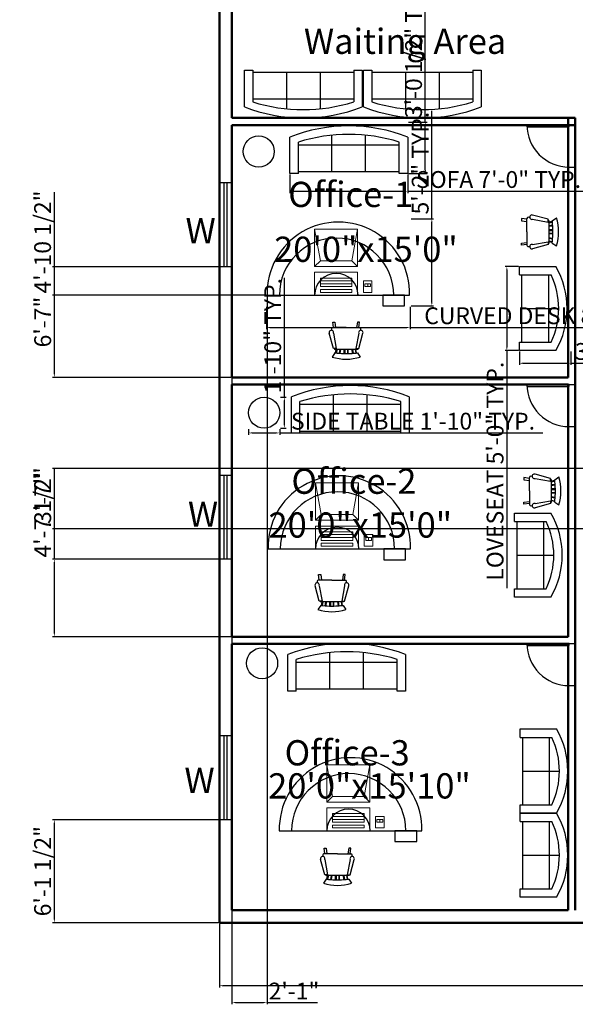
# Model space of a CAD drawing. Units: inches. Extents: x 1953 to 3378, y 1378 to 2530.
# Tile 1 of 5: x 1953 to 2350, y 1388 to 2090. Entities that reach past the tile are written whole.
import ezdxf

# ---------------------------------------------------------------- set-up
doc = ezdxf.new("R2010")
doc.units = ezdxf.units.IN
for name, color, linetype, lineweight in [('A-ANNO-DIMS', 2, 'Continuous', 18), ('A-ANNO-TEXT', 7, 'Continuous', 18), ('A-AREA-IDEN', 4, 'Continuous', 18), ('A-DOOR', 4, 'Continuous', 25), ('A-EQPM', 50, 'Continuous', 18), ('A-FURN', 50, 'Continuous', 25), ('wall', 7, 'Continuous', 50), ('windows', 180, 'Continuous', 25)]:
    doc.layers.add(name, color=color, linetype=linetype, lineweight=lineweight)
doc.styles.get("Standard").update_dxf_attribs({"font": 'arial.ttf'})
doc.dimstyles.new('ISO-25', dxfattribs={"dimtxt": 12, "dimasz": 2.5, "dimexe": 1.25, "dimexo": 0.625, "dimtad": 1, "dimdec": 1, "dimlunit": 4, "dimtxsty": 'Standard', "dimcen": 2.5, "dimadec": 0, "dimazin": 0, "dimtfac": 1, "dimtdec": 1, "dimtmove": 0, "dimatfit": 3, "dimfxl": 1, "dimarcsym": 0})

# ---------------------------------------------------------------- blocks, each defined once
blk = doc.blocks.new('*U10')
for p, q in [((0, 0), (0, 6)), ((40, 0), (40, 6))]:
    blk.add_line(p, q)
blk.add_lwpolyline([(0, 0), (0, -40), (1.75, -40), (1.75, 0)], close=True)
blk.add_arc((0, 0), 40, 270, 0)
blk = doc.blocks.new('*U9')
for p, q in [((0, 0), (0, 6)), ((40, 0), (40, 6))]:
    blk.add_line(p, q)
blk.add_lwpolyline([(0, 0), (0, -40), (1.75, -40), (1.75, 0)], close=True)
blk.add_arc((0, 0), 40, 270, 0)
blk = doc.blocks.new('*U8')
for p, q in [((0, 0), (0, 6)), ((40, 0), (40, 6))]:
    blk.add_line(p, q)
blk.add_lwpolyline([(0, 0), (0, -40), (1.75, -40), (1.75, 0)], close=True)
blk.add_arc((0, 0), 40, 270, 360)
blk = doc.blocks.new('Sofa - Roundback 7 ft.')
for p, q in [((-12.00002, -32.4421), (-12.00003, -6.5971)), ((11.99997, -32.4421), (11.99998, -6.5971)), ((-36.000027, -34), (-36.000027, -11.4696)), ((-35.999844, -13.3819), (35.9998, -13.3819)), ((35.99998, -34), (35.99998, -11.4696)), ((-36.000027, -32.4421), (35.99998, -32.4421))]:
    blk.add_line(p, q)
for points in [[(-36.000027, -34), (-42.000027, -34), (-42.000027, -8)], [(41.99998, -8), (41.99998, -34), (35.99998, -34)]]:
    blk.add_lwpolyline(points)
for centre, radius, start, end in [((0, -114.25), 114.25, 68.43141, 111.5686), ((-0.00001, -127.1968), 121.1968, 72.72033, 107.2797)]:
    blk.add_arc(centre, radius, start, end)
blk = doc.blocks.new('Computer Terminal')
for p, q in [((-10, 11.5), (5, 11.5)), ((-8, 0.5), (-10, 11.5)), ((-10, -1.5), (-10, 11.5)), ((5, 11.5), (3, 0.5)), ((5, 11.5), (5, -1.5)), ((-10, -1.5), (-8, 0.5)), ((3, 0.5), (-8, 0.5)), ((3, 0.5), (5, -1.5)), ((5, -1.5), (-10, -1.5)), ((-10, -11.5), (-10, -3.5)), ((-10, -3.5), (5, -3.5)), ((-8, -5.5), (-8, -8.5)), ((3, -5.5), (-8, -5.5)), ((3, -6.5), (-8, -6.5)), ((3, -8.5), (3, -5.5)), ((5, -3.5), (5, -11.5)), ((10, -6.5), (7, -6.5)), ((7, -6.5), (7, -10.5)), ((10, -10.5), (10, -6.5)), ((-8, -7.5), (3, -7.5)), ((-8, -8.5), (3, -8.5)), ((-8, -9.5), (-8, -10.5)), ((3, -9.5), (-8, -9.5)), ((3, -10.5), (3, -9.5)), ((9.5, -7.5), (7.5, -7.5)), ((7.5, -7.5), (7.5, -8.5)), ((7.5, -8.5), (9.5, -8.5)), ((8.5, -7.5), (8.5, -8.5)), ((9.5, -8.5), (9.5, -7.5)), ((5, -11.5), (-10, -11.5)), ((-8, -10.5), (3, -10.5)), ((7, -10.5), (10, -10.5))]:
    blk.add_line(p, q)
blk = doc.blocks.new('Chair - Rocking')
for p, q in [((-8, -4.5), (-10, -1.5)), ((-8.23428, -6.99939), (-8.3093, -7.47958)), ((-8.23041, -7), (8.23915, -7)), ((-7.5, -4.5), (-7, -7)), ((-6.5, -7), (-7.02225, -4.43)), ((-4.5, -7), (-4.96674, -4.19951)), ((-4, -7), (-4.40532, -4.16272)), ((-1.5, -4.05012), (-1.5, -7)), ((-1, -7), (-1, -4.05012)), ((1, -7), (1, -4.04655)), ((1.5, -4.05012), (1.5, -7)), ((4, -7), (4.40187, -4.18694)), ((4.5, -7), (4.96761, -4.19437)), ((6.5, -7), (7, -4.4057)), ((7.5, -4.5), (7, -7)), ((8, -4.5), (10, -1.5)), ((8.31071, -7.48854), (8.23449, -7.00073)), ((-9, -7.5), (-12, -18.49999)), ((-7, -7.5), (-9, -7.5)), ((-9, -18.49999), (-7, -7.5)), ((7, -7.5), (9, -7.5)), ((9, -18.49999), (7, -7.5)), ((9, -7.5), (12, -18.49999)), ((-10.36644, -20.64523), (-10.5, -21.49999)), ((10.5, -21.49999), (10.3575, -20.58798)), ((-9, -22.49999), (-9.5, -26.49999)), ((0, -22.49999), (-9.5, -22.49999)), ((-9.5, -26.49999), (-8, -26.49999)), ((-8, -26.49999), (-7.5, -22.49999)), ((0, -22.49999), (9.5, -22.49999)), ((8, -26.49999), (7.5, -22.49999)), ((9.5, -26.49999), (8, -26.49999)), ((9, -22.49999), (9.5, -26.49999))]:
    blk.add_line(p, q)
for centre, radius, start, end in [((0, -34.08333), 34.08333, 72.93847, 107.0615), ((0, -68.25004), 64.25, 93.92211, 97.15267), ((0, -68.25004), 64.25, 82.84733, 93.92211), ((-10.5, -18.99999), 1.58114, 161.5651, 18.43495), ((10.5, -18.99999), 1.58114, 161.5651, 18.43495), ((-9.5, -21.49999), 1, 180, 270), ((9.5, -21.49999), 1, 270, 0)]:
    blk.add_arc(centre, radius, start, end)
blk = doc.blocks.new('Sofa - Roundback Loveseat 5 ft.')
for p, q in [((0, -32.44198), (0, -5.99998)), ((-24, -33.99998), (-24, -11.46958)), ((-23.9998, -13.38178), (23.99986, -13.38178)), ((24.00004, -33.99998), (24.00004, -11.46958)), ((-24, -32.44198), (24.00004, -32.44198))]:
    blk.add_line(p, q)
for points in [[(-24, -33.99998), (-30, -33.99998), (-30, -7.99998)], [(30.00004, -7.99998), (30.00004, -33.99998), (24.00004, -33.99998)]]:
    blk.add_lwpolyline(points)
for centre, radius, start, end in [((0, -60.24998), 60.24998, 60.13715, 119.8628), ((0, -61.38438), 55.38444, 64.32083, 115.6792)]:
    blk.add_arc(centre, radius, start, end)
blk = doc.blocks.new('*D28')
at = {"layer": 'A-ANNO-DIMS', "color": 0, "lineweight": -2, "transparency": 16777216}
for p, q in [((2095.75, 1445.39), (2095.75, 1399.8)), ((2695.75, 1445.39), (2695.75, 1399.8)), ((2693.25, 1401.05), (2098.25, 1401.05))]:
    blk.add_line(p, q, dxfattribs=at)
at = {"layer": 'A-ANNO-DIMS', "color": 0, "transparency": 16777216}
for points in [[(2098.25, 1401.47), (2098.25, 1400.63), (2095.75, 1401.05)], [(2693.25, 1401.47), (2693.25, 1400.63), (2695.75, 1401.05)]]:
    blk.add_solid(points, dxfattribs=at)
at = {"layer": 'Defpoints', "color": 0, "transparency": 16777216}
for p in [(2095.75, 1446.01), (2695.75, 1446.01), (2095.75, 1401.05)]:
    blk.add_point(p, dxfattribs=at)
at = {"layer": 'A-ANNO-DIMS', "color": 0, "transparency": 16777216, "insert": (2395.75, 1407.8), "char_height": 12, "attachment_point": 5}
blk.add_mtext("50'", dxfattribs=at)
blk = doc.blocks.new('WINDOW-60IN')
for p, q in [((0, 5.5), (60, 5.5)), ((0, 5.5), (60, 5.5)), ((0, 3.5), (60, 3.5))]:
    blk.add_line(p, q)
blk.add_lwpolyline([(0, 9), (60, 9), (60, 0), (0, 0)], close=True)
blk = doc.blocks.new('DESK-SEMICIRCULAR')
blk.add_line((0.02, 7.63), (101.66, 7.63))
blk.add_lwpolyline([(82.57, 7.63), (82.57, 0), (98.08, 0), (98.08, 7.63)], close=True)
for centre, radius, start, end in [((50.84, 8.97), 50.84, 358.48644, 181.51356), ((49.55, 7.63), 40.78, 0, 180), ((49.41, 7.63), 15.51, 0, 180)]:
    blk.add_arc(centre, radius, start, end)
blk = doc.blocks.new('SIDE-TABLE-ROUND')
blk.add_circle((11.1, 11.1), 11.1)
blk = doc.blocks.new('*D40')
at = {"layer": 'A-ANNO-DIMS', "color": 0, "lineweight": -2, "transparency": 16777216}
for p, q in [((2309.27, 1914.09), (2299.64, 1914.09)), ((2300.89, 1911.59), (2300.89, 1856.59)), ((2309.27, 1854.09), (2299.64, 1854.09)), ((2300.89, 1854.09), (2300.89, 1684.55))]:
    blk.add_line(p, q, dxfattribs=at)
at = {"layer": 'A-ANNO-DIMS', "color": 0, "transparency": 16777216}
for points in [[(2300.47, 1911.59), (2301.31, 1911.59), (2300.89, 1914.09)], [(2300.47, 1856.59), (2301.31, 1856.59), (2300.89, 1854.09)]]:
    blk.add_solid(points, dxfattribs=at)
at = {"layer": 'Defpoints', "color": 0, "transparency": 16777216}
for p in [(2309.89, 1914.09), (2300.89, 1854.09), (2309.89, 1854.09)]:
    blk.add_point(p, dxfattribs=at)
at = {"layer": 'A-ANNO-DIMS', "color": 0, "transparency": 16777216, "insert": (2294.06, 1768.07), "char_height": 12, "attachment_point": 5, "rotation": 90}
blk.add_mtext('LOVESEAT 5\'-0" TYP.', dxfattribs=at)
blk = doc.blocks.new('*D41')
at = {"layer": 'A-ANNO-DIMS', "color": 0, "lineweight": -2, "transparency": 16777216}
for p, q in [((2309.89, 1853.46), (2309.89, 1843.84)), ((2346.56, 1853.46), (2346.56, 1843.84)), ((2312.39, 1845.09), (2344.06, 1845.09)), ((2346.56, 1845.09), (2451.41, 1845.09))]:
    blk.add_line(p, q, dxfattribs=at)
at = {"layer": 'A-ANNO-DIMS', "color": 0, "transparency": 16777216}
for points in [[(2312.39, 1845.5), (2312.39, 1844.67), (2309.89, 1845.09)], [(2344.06, 1845.5), (2344.06, 1844.67), (2346.56, 1845.09)]]:
    blk.add_solid(points, dxfattribs=at)
at = {"layer": 'Defpoints', "color": 0, "transparency": 16777216}
for p in [(2309.89, 1854.09), (2346.56, 1854.09), (2346.56, 1845.09)]:
    blk.add_point(p, dxfattribs=at)
at = {"layer": 'A-ANNO-DIMS', "color": 0, "transparency": 16777216, "insert": (2400.23, 1851.92), "char_height": 12, "attachment_point": 5}
blk.add_mtext('3\'-0 1/2" TYP.', dxfattribs=at)
blk = doc.blocks.new('*D42')
at = {"layer": 'A-ANNO-DIMS', "color": 0, "lineweight": -2, "transparency": 16777216}
for p, q in [((2146.13, 1979.72), (2146.13, 1966.49)), ((2230.13, 1979.72), (2230.13, 1966.49)), ((2148.63, 1967.74), (2227.63, 1967.74)), ((2230.13, 1967.74), (2357.26, 1967.74))]:
    blk.add_line(p, q, dxfattribs=at)
at = {"layer": 'A-ANNO-DIMS', "color": 0, "transparency": 16777216}
for points in [[(2148.63, 1968.16), (2148.63, 1967.33), (2146.13, 1967.74)], [(2227.63, 1968.16), (2227.63, 1967.33), (2230.13, 1967.74)]]:
    blk.add_solid(points, dxfattribs=at)
at = {"layer": 'Defpoints', "color": 0, "transparency": 16777216}
for p in [(2146.13, 1980.34), (2230.13, 1980.34), (2230.13, 1967.74)]:
    blk.add_point(p, dxfattribs=at)
at = {"layer": 'A-ANNO-DIMS', "color": 0, "transparency": 16777216, "insert": (2294.95, 1974.58), "char_height": 12, "attachment_point": 5}
blk.add_mtext('SOFA 7\'-0" TYP.', dxfattribs=at)
blk = doc.blocks.new('*D43')
at = {"layer": 'A-ANNO-DIMS', "color": 0, "lineweight": -2, "transparency": 16777216}
for p, q in [((2242.73, 2017.01), (2242.73, 2121.86)), ((2230.75, 2017.01), (2243.98, 2017.01)), ((2242.73, 1982.84), (2242.73, 2014.51)), ((2230.75, 1980.34), (2243.98, 1980.34))]:
    blk.add_line(p, q, dxfattribs=at)
at = {"layer": 'A-ANNO-DIMS', "color": 0, "transparency": 16777216}
for points in [[(2242.31, 2014.51), (2243.14, 2014.51), (2242.73, 2017.01)], [(2242.31, 1982.84), (2243.14, 1982.84), (2242.73, 1980.34)]]:
    blk.add_solid(points, dxfattribs=at)
at = {"layer": 'Defpoints', "color": 0, "transparency": 16777216}
for p in [(2230.13, 2017.01), (2242.73, 2017.01), (2230.13, 1980.34)]:
    blk.add_point(p, dxfattribs=at)
at = {"layer": 'A-ANNO-DIMS', "color": 0, "transparency": 16777216, "insert": (2235.89, 2070.69), "char_height": 12, "attachment_point": 5, "rotation": 90}
blk.add_mtext('3\'-0 1/2" TYP.', dxfattribs=at)
blk = doc.blocks.new('*D44')
at = {"layer": 'A-ANNO-DIMS', "color": 0, "lineweight": -2, "transparency": 16777216}
for p, q in [((2129.36, 1885.33), (2129.36, 1869.31)), ((2231.98, 1885.33), (2231.98, 1869.31)), ((2131.86, 1870.56), (2229.48, 1870.56)), ((2231.98, 1870.56), (2462.45, 1870.56))]:
    blk.add_line(p, q, dxfattribs=at)
at = {"layer": 'A-ANNO-DIMS', "color": 0, "transparency": 16777216}
for points in [[(2131.86, 1870.98), (2131.86, 1870.14), (2129.36, 1870.56)], [(2229.48, 1870.98), (2229.48, 1870.14), (2231.98, 1870.56)]]:
    blk.add_solid(points, dxfattribs=at)
at = {"layer": 'Defpoints', "color": 0, "transparency": 16777216}
for p in [(2129.36, 1885.95), (2231.98, 1885.95), (2231.98, 1870.56)]:
    blk.add_point(p, dxfattribs=at)
at = {"layer": 'A-ANNO-DIMS', "color": 0, "transparency": 16777216, "insert": (2348.46, 1877.39), "char_height": 12, "attachment_point": 5}
blk.add_mtext('CURVED DESK 8\'-6 1/2" TYP.', dxfattribs=at)
blk = doc.blocks.new('*D45')
at = {"layer": 'A-ANNO-DIMS', "color": 0, "lineweight": -2, "transparency": 16777216}
for p, q in [((2247.37, 1948.11), (2247.37, 2025.01)), ((2232.6, 1948.11), (2248.62, 1948.11)), ((2247.37, 1888.45), (2247.37, 1945.61)), ((2232.6, 1885.95), (2248.62, 1885.95))]:
    blk.add_line(p, q, dxfattribs=at)
at = {"layer": 'A-ANNO-DIMS', "color": 0, "transparency": 16777216}
for points in [[(2246.96, 1945.61), (2247.79, 1945.61), (2247.37, 1948.11)], [(2246.96, 1888.45), (2247.79, 1888.45), (2247.37, 1885.95)]]:
    blk.add_solid(points, dxfattribs=at)
at = {"layer": 'Defpoints', "color": 0, "transparency": 16777216}
for p in [(2231.98, 1948.11), (2247.37, 1948.11), (2231.98, 1885.95)]:
    blk.add_point(p, dxfattribs=at)
at = {"layer": 'A-ANNO-DIMS', "color": 0, "transparency": 16777216, "insert": (2240.62, 1987.81), "char_height": 12, "attachment_point": 5, "rotation": 90}
blk.add_mtext('5\'-2" TYP.', dxfattribs=at)
blk = doc.blocks.new('*D48')
at = {"layer": 'A-ANNO-DIMS', "color": 0, "lineweight": -2, "transparency": 16777216}
for p, q in [((2116.61, 1798.07), (2116.61, 1794.11)), ((2138.81, 1798.07), (2138.81, 1794.11)), ((2119.11, 1795.36), (2136.31, 1795.36)), ((2138.81, 1795.36), (2326.52, 1795.36))]:
    blk.add_line(p, q, dxfattribs=at)
at = {"layer": 'A-ANNO-DIMS', "color": 0, "transparency": 16777216}
for points in [[(2119.11, 1795.78), (2119.11, 1794.95), (2116.61, 1795.36)], [(2136.31, 1795.78), (2136.31, 1794.95), (2138.81, 1795.36)]]:
    blk.add_solid(points, dxfattribs=at)
at = {"layer": 'Defpoints', "color": 0, "transparency": 16777216}
for p in [(2116.61, 1798.69), (2138.81, 1798.69), (2138.81, 1795.36)]:
    blk.add_point(p, dxfattribs=at)
at = {"layer": 'A-ANNO-DIMS', "color": 0, "transparency": 16777216, "insert": (2233.92, 1802.19), "char_height": 12, "attachment_point": 5}
blk.add_mtext('SIDE TABLE 1\'-10" TYP.', dxfattribs=at)
blk = doc.blocks.new('*D49')
at = {"layer": 'A-ANNO-DIMS', "color": 0, "lineweight": -2, "transparency": 16777216}
for p, q in [((2142.14, 1820.89), (2142.14, 1905.98)), ((2139.44, 1820.89), (2143.39, 1820.89)), ((2142.14, 1801.19), (2142.14, 1818.39)), ((2139.44, 1798.69), (2143.39, 1798.69))]:
    blk.add_line(p, q, dxfattribs=at)
at = {"layer": 'A-ANNO-DIMS', "color": 0, "transparency": 16777216}
for points in [[(2141.72, 1818.39), (2142.56, 1818.39), (2142.14, 1820.89)], [(2141.72, 1801.19), (2142.56, 1801.19), (2142.14, 1798.69)]]:
    blk.add_solid(points, dxfattribs=at)
at = {"layer": 'Defpoints', "color": 0, "transparency": 16777216}
for p in [(2138.81, 1820.89), (2142.14, 1820.89), (2138.81, 1798.69)]:
    blk.add_point(p, dxfattribs=at)
at = {"layer": 'A-ANNO-DIMS', "color": 0, "transparency": 16777216, "insert": (2135.39, 1864.69), "char_height": 12, "attachment_point": 5, "rotation": 90}
blk.add_mtext('1\'-10" TYP.', dxfattribs=at)
blk = doc.blocks.new('*D66')
at = {"layer": 'A-ANNO-DIMS', "color": 0, "lineweight": -2, "transparency": 16777216}
for p, q in [((2095.12, 1519.49), (1976.77, 1519.49)), ((1978.02, 1448.51), (1978.02, 1516.99)), ((2095.12, 1446.01), (1976.77, 1446.01))]:
    blk.add_line(p, q, dxfattribs=at)
at = {"layer": 'A-ANNO-DIMS', "color": 0, "transparency": 16777216}
for points in [[(1977.6, 1516.99), (1978.44, 1516.99), (1978.02, 1519.49)], [(1977.6, 1448.51), (1978.44, 1448.51), (1978.02, 1446.01)]]:
    blk.add_solid(points, dxfattribs=at)
at = {"layer": 'Defpoints', "color": 0, "transparency": 16777216}
for p in [(1978.02, 1519.49), (2095.75, 1519.49), (2095.75, 1446.01)]:
    blk.add_point(p, dxfattribs=at)
at = {"layer": 'A-ANNO-DIMS', "color": 0, "transparency": 16777216, "insert": (1971.19, 1482.75), "char_height": 12, "attachment_point": 5, "rotation": 90}
blk.add_mtext('6\'-1 1/2"', dxfattribs=at)
blk = doc.blocks.new('*D67')
at = {"layer": 'A-ANNO-DIMS', "color": 0, "lineweight": -2, "transparency": 16777216}
for p, q in [((1978.02, 1705.35), (1978.02, 1769.45)), ((2104.12, 1705.35), (1976.77, 1705.35)), ((1978.02, 1652.51), (1978.02, 1702.85)), ((2104.12, 1650.01), (1976.77, 1650.01))]:
    blk.add_line(p, q, dxfattribs=at)
at = {"layer": 'A-ANNO-DIMS', "color": 0, "transparency": 16777216}
for points in [[(1977.6, 1702.85), (1978.44, 1702.85), (1978.02, 1705.35)], [(1977.6, 1652.51), (1978.44, 1652.51), (1978.02, 1650.01)]]:
    blk.add_solid(points, dxfattribs=at)
at = {"layer": 'Defpoints', "color": 0, "transparency": 16777216}
for p in [(1978.02, 1705.35), (2104.75, 1705.35), (2104.75, 1650.01)]:
    blk.add_point(p, dxfattribs=at)
at = {"layer": 'A-ANNO-DIMS', "color": 0, "transparency": 16777216, "insert": (1971.19, 1738.65), "char_height": 12, "attachment_point": 5, "rotation": 90}
blk.add_mtext('4\'-7 1/2"', dxfattribs=at)
blk = doc.blocks.new('*D68')
at = {"layer": 'A-ANNO-DIMS', "color": 0, "lineweight": -2, "transparency": 16777216}
for p, q in [((2104.12, 1913.91), (1976.77, 1913.91)), ((1978.02, 1837.51), (1978.02, 1911.41)), ((2104.12, 1835.01), (1976.77, 1835.01))]:
    blk.add_line(p, q, dxfattribs=at)
at = {"layer": 'A-ANNO-DIMS', "color": 0, "transparency": 16777216}
for points in [[(1977.6, 1911.41), (1978.44, 1911.41), (1978.02, 1913.91)], [(1977.6, 1837.51), (1978.44, 1837.51), (1978.02, 1835.01)]]:
    blk.add_solid(points, dxfattribs=at)
at = {"layer": 'Defpoints', "color": 0, "transparency": 16777216}
for p in [(1978.02, 1913.91), (2104.75, 1913.91), (2104.75, 1835.01)]:
    blk.add_point(p, dxfattribs=at)
at = {"layer": 'A-ANNO-DIMS', "color": 0, "transparency": 16777216, "insert": (1971.27, 1874.46), "char_height": 12, "attachment_point": 5, "rotation": 90}
blk.add_mtext('6\'-7"', dxfattribs=at)
blk = doc.blocks.new('*D83')
at = {"layer": 'A-ANNO-DIMS', "color": 0, "lineweight": -2, "transparency": 16777216}
for p, q in [((2462.77, 1770), (1976.77, 1770)), ((1978.02, 1729.51), (1978.02, 1767.5)), ((2441.12, 1727.01), (1976.77, 1727.01))]:
    blk.add_line(p, q, dxfattribs=at)
at = {"layer": 'A-ANNO-DIMS', "color": 0, "transparency": 16777216}
for points in [[(1977.6, 1767.5), (1978.44, 1767.5), (1978.02, 1770)], [(1977.6, 1729.51), (1978.44, 1729.51), (1978.02, 1727.01)]]:
    blk.add_solid(points, dxfattribs=at)
at = {"layer": 'Defpoints', "color": 0, "transparency": 16777216}
for p in [(1978.02, 1770), (2463.39, 1770), (2441.75, 1727.01)]:
    blk.add_point(p, dxfattribs=at)
at = {"layer": 'A-ANNO-DIMS', "color": 0, "transparency": 16777216, "insert": (1971.26, 1748.51), "char_height": 12, "attachment_point": 5, "rotation": 90}
blk.add_mtext('3\'-7"', dxfattribs=at)
blk = doc.blocks.new('*D86')
at = {"layer": 'A-ANNO-DIMS', "color": 0, "lineweight": -2, "transparency": 16777216}
for p, q in [((2129.84, 1892.96), (2129.84, 1387.78)), ((2104.75, 1834.39), (2104.75, 1387.78)), ((2107.25, 1389.03), (2127.34, 1389.03)), ((2129.84, 1389.03), (2165.7, 1389.03))]:
    blk.add_line(p, q, dxfattribs=at)
at = {"layer": 'A-ANNO-DIMS', "color": 0, "transparency": 16777216}
for points in [[(2107.25, 1389.45), (2107.25, 1388.62), (2104.75, 1389.03)], [(2127.34, 1389.45), (2127.34, 1388.62), (2129.84, 1389.03)]]:
    blk.add_solid(points, dxfattribs=at)
at = {"layer": 'Defpoints', "color": 0, "transparency": 16777216}
for p in [(2129.84, 1893.58), (2104.75, 1835.01), (2129.84, 1389.03)]:
    blk.add_point(p, dxfattribs=at)
at = {"layer": 'A-ANNO-DIMS', "color": 0, "transparency": 16777216, "insert": (2149.02, 1395.68), "char_height": 12, "attachment_point": 5}
blk.add_mtext('2\'-1"', dxfattribs=at)
blk = doc.blocks.new('*D87')
at = {"layer": 'A-ANNO-DIMS', "color": 0, "lineweight": -2, "transparency": 16777216}
for p, q in [((1978.02, 1893.58), (1978.02, 1967)), ((2129.22, 1893.58), (1976.77, 1893.58)), ((1978.02, 1837.51), (1978.02, 1891.08)), ((2104.12, 1835.01), (1976.77, 1835.01))]:
    blk.add_line(p, q, dxfattribs=at)
at = {"layer": 'A-ANNO-DIMS', "color": 0, "transparency": 16777216}
for points in [[(1977.6, 1891.08), (1978.44, 1891.08), (1978.02, 1893.58)], [(1977.6, 1837.51), (1978.44, 1837.51), (1978.02, 1835.01)]]:
    blk.add_solid(points, dxfattribs=at)
at = {"layer": 'Defpoints', "color": 0, "transparency": 16777216}
for p in [(1978.02, 1893.58), (2129.84, 1893.58), (2104.75, 1835.01)]:
    blk.add_point(p, dxfattribs=at)
at = {"layer": 'A-ANNO-DIMS', "color": 0, "transparency": 16777216, "insert": (1971.19, 1931.54), "char_height": 12, "attachment_point": 5, "rotation": 90}
blk.add_mtext('4\'-10 1/2"', dxfattribs=at)

msp = doc.modelspace()

# ---------------------------------------------------------------- linework, layer by layer
at = {"layer": 'wall'}
for p, q in [((2095.75, 1446.01), (2095.75, 2286.01)), ((2104.75, 2020.01), (2104.75, 2277.01)), ((2104.75, 2020.01), (2349.75, 2020.01)), ((2344.75, 1835.01), (2344.75, 2020.01)), ((2349.75, 1455.01), (2349.75, 2020.01)), ((2104.75, 2015.01), (2349.75, 2015.01)), ((2104.75, 1835.01), (2104.75, 2015.01)), ((2104.75, 1835.01), (2344.75, 1835.01)), ((2104.75, 1830.01), (2344.75, 1830.01)), ((2104.75, 1650.01), (2104.75, 1830.01)), ((2344.75, 1650.01), (2344.75, 1830.01)), ((2104.75, 1650.01), (2344.75, 1650.01)), ((2104.75, 1455.01), (2104.75, 1645.01)), ((2104.75, 1645.01), (2344.75, 1645.01)), ((2344.75, 1455.01), (2344.75, 1645.01)), ((2344.75, 1455.01), (2104.75, 1455.01)), ((2695.75, 1446.01), (2095.75, 1446.01))]:
    msp.add_line(p, q, dxfattribs=at)

# ---------------------------------------------------------------- block references
at = {"layer": 'A-DOOR', "xscale": 0.75, "yscale": 0.75, "zscale": 0.75, "rotation": 270}
for name, p in [('*U10', (2345.25, 2015.01)), ('*U9', (2345.25, 1829.9)), ('*U8', (2345.25, 1645.14))]:
    msp.add_blockref(name, p, dxfattribs=at)
at = {"layer": 'A-EQPM', "xscale": 2.047281239074101, "yscale": 2.047281239074101, "zscale": 2.047281239074101}
for p in [(2184.2, 1917.13), (2184.83, 1736.11), (2192.88, 1535.07)]:
    msp.add_blockref('Computer Terminal', p, dxfattribs=at)
at = {"layer": 'A-FURN'}
for name, p, rotation in [('Sofa - Roundback 7 ft.', (2155.62, 2020.01), 180), ('Sofa - Roundback 7 ft.', (2240.53, 2020.01), 180), ('Chair - Rocking', (2337.77, 1938.77), 270), ('Sofa - Roundback Loveseat 5 ft.', (2343.89, 1884.09), 269.9999999999999), ('Chair - Rocking', (2186.23, 1847.97), 180), ('Chair - Rocking', (2339.53, 1753.96), 270), ('Sofa - Roundback Loveseat 5 ft.', (2340.39, 1708.21), 269.9999999999999), ('Chair - Rocking', (2176.06, 1667.85), 180), ('Sofa - Roundback Loveseat 5 ft.', (2344.41, 1554.17), 269.9999999999999), ('Sofa - Roundback Loveseat 5 ft.', (2344.41, 1494.17), 269.9999999999999), ('Chair - Rocking', (2180.04, 1472.6), 180)]:
    msp.add_blockref(name, p, dxfattribs=dict(at, rotation=rotation))
for name, p in [('Sofa - Roundback 7 ft.', (2188.13, 2014.34)), ('SIDE-TABLE-ROUND', (2112.72, 1985)), ('DESK-SEMICIRCULAR', (2129.83, 1885.95)), ('Sofa - Roundback 7 ft.', (2189.28, 1829.17)), ('SIDE-TABLE-ROUND', (2116.61, 1798.69)), ('DESK-SEMICIRCULAR', (2130.46, 1704.94)), ('Sofa - Roundback 7 ft.', (2186.68, 1645.25)), ('SIDE-TABLE-ROUND', (2115.17, 1619.97)), ('DESK-SEMICIRCULAR', (2138.51, 1503.9))]:
    msp.add_blockref(name, p, dxfattribs=at)
at = {"layer": 'windows'}
for p, rotation in [((2104.75, 1913.91), 90.00000000000078), ((2104.75, 1705.35), 90.00000000000055), ((2104.75, 1519.49), 90.00000000000063)]:
    msp.add_blockref('WINDOW-60IN', p, dxfattribs=dict(at, rotation=rotation))

# ---------------------------------------------------------------- texts
at = {"layer": 'A-ANNO-TEXT'}
for p in [(2071.64, 1930.57), (2073.34, 1728.39), (2070.85, 1538.5)]:
    msp.add_text('W', height=18, dxfattribs=at).set_placement(p)
at = {"layer": 'A-AREA-IDEN'}
for s, p in [('Waiting Area', (2156.1, 2065.73)), ('Office-1', (2144.89, 1956.51)), ('20\'0"x15\'0"', (2134.9, 1917.37)), ('Office-2', (2147.19, 1751.92)), ('20\'0"x15\'0"', (2130.87, 1720.67)), ('Office-3', (2142.35, 1558.2)), ('20\'0"x15\'10"', (2130.57, 1534.59))]:
    msp.add_text(s, height=18, dxfattribs=at).set_placement(p)

# ---------------------------------------------------------------- dimensions: what is measured, and where the dimension line sits
at = {"layer": 'A-ANNO-DIMS'}
for base, p1, p2, angle, text, picture, middle in [((2242.73, 2017.01), (2230.13, 1980.34), (2230.13, 2017.01), 90, '<> TYP.', '*D43', (2235.89, 2070.69)), ((2247.37, 1948.11), (2231.98, 1885.95), (2231.98, 1948.11), 90, '<> TYP.', '*D45', (2240.62, 1987.81)), ((2300.89, 1854.09), (2309.89, 1914.09), (2309.89, 1854.09), 270, 'LOVESEAT <> TYP.', '*D40', (2294.06, 1768.07)), ((2142.14, 1820.89), (2138.81, 1798.69), (2138.81, 1820.89), 90, '<> TYP.', '*D49', (2135.39, 1864.69))]:
    dim = msp.add_linear_dim(base=base, p1=p1, p2=p2, angle=angle, text=text, dimstyle='ISO-25', override={"dimdec": 1, "dimlfac": 1, "dimrnd": 0, "dimzin": 1, "dimdsep": 46, "dimlunit": 4, "dimfrac": 2}, dxfattribs=at)
    dim.commit()
    dim.dimension.update_dxf_attribs({"geometry": picture, "text_midpoint": middle})
for base, p1, p2, text, picture, middle in [((2230.13, 1967.74), (2146.13, 1980.34), (2230.13, 1980.34), 'SOFA <> TYP.', '*D42', (2294.95, 1974.58)), ((2231.98, 1870.56), (2129.36, 1885.95), (2231.98, 1885.95), 'CURVED DESK <> TYP.', '*D44', (2348.46, 1877.39)), ((2346.56, 1845.09), (2309.89, 1854.09), (2346.56, 1854.09), '<> TYP.', '*D41', (2400.23, 1851.92)), ((2138.81, 1795.36), (2116.61, 1798.69), (2138.81, 1798.69), 'SIDE TABLE <> TYP.', '*D48', (2233.92, 1802.19))]:
    dim = msp.add_linear_dim(base=base, p1=p1, p2=p2, text=text, dimstyle='ISO-25', override={"dimdec": 1, "dimlfac": 1, "dimrnd": 0, "dimzin": 1, "dimdsep": 46, "dimlunit": 4, "dimfrac": 2}, dxfattribs=at)
    dim.commit()
    dim.dimension.update_dxf_attribs({"geometry": picture, "text_midpoint": middle})
for base, p1, p2, picture, middle in [((1978.02, 1893.58), (2104.75, 1835.01), (2129.84, 1893.58), '*D87', (1971.19, 1931.54)), ((1978.02, 1913.91), (2104.75, 1835.01), (2104.75, 1913.91), '*D68', (1971.27, 1874.46)), ((1978.02, 1770), (2441.75, 1727.01), (2463.39, 1770), '*D83', (1971.26, 1748.51)), ((1978.02, 1705.35), (2104.75, 1650.01), (2104.75, 1705.35), '*D67', (1971.19, 1738.65)), ((1978.02, 1519.49), (2095.75, 1446.01), (2095.75, 1519.49), '*D66', (1971.19, 1482.75))]:
    dim = msp.add_linear_dim(base=base, p1=p1, p2=p2, angle=90, dimstyle='ISO-25', override={"dimdec": 1, "dimlfac": 1, "dimrnd": 0, "dimzin": 1, "dimdsep": 46, "dimlunit": 4, "dimfrac": 2}, dxfattribs=at)
    dim.commit()
    dim.dimension.update_dxf_attribs({"geometry": picture, "text_midpoint": middle})
for base, p1, p2, override, picture, middle in [((2129.84, 1389.03), (2104.75, 1835.01), (2129.84, 1893.58), {"dimdec": 1, "dimlfac": 1, "dimrnd": 0, "dimzin": 1, "dimdsep": 46, "dimlunit": 4, "dimfrac": 2}, '*D86', (2149.02, 1395.68)), ((2095.75, 1401.05), (2695.75, 1446.01), (2095.75, 1446.01), {"dimclrd": 0, "dimclre": 0, "dimclrt": 0}, '*D28', (2395.75, 1407.8))]:
    dim = msp.add_linear_dim(base=base, p1=p1, p2=p2, dimstyle='ISO-25', override=override, dxfattribs=at)
    dim.commit()
    dim.dimension.update_dxf_attribs({"geometry": picture, "text_midpoint": middle})

doc.saveas('drawing.dxf')
